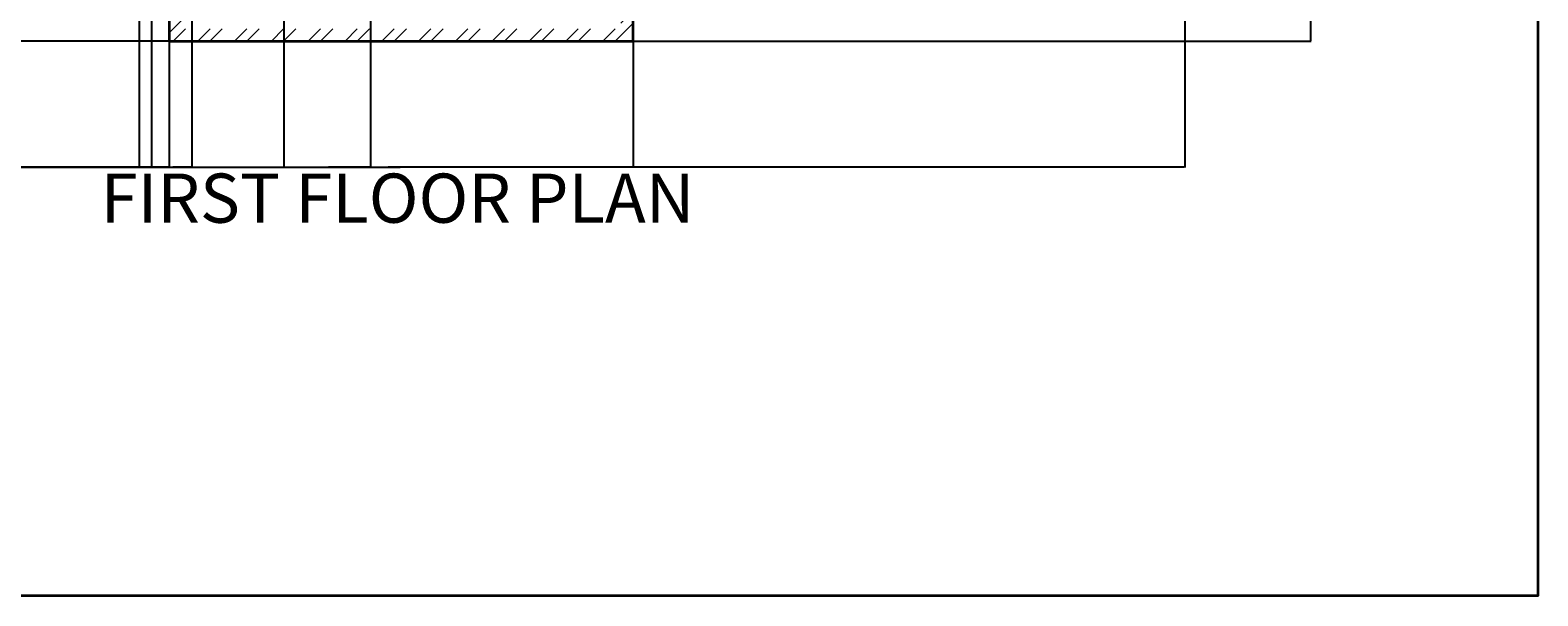
# Model space of a CAD drawing. Units: inches. Extents: x 392 to 1254, y 1207 to 2665.
# Tile 2 of 15: x 702 to 1254, y 1207 to 1414. Entities that reach past the tile are written whole.
import ezdxf

# ---------------------------------------------------------------- set-up
doc = ezdxf.new("R2010")
doc.units = ezdxf.units.IN
for name, color, linetype, lineweight in [('A-ANNO-DIMS', 2, 'Continuous', 18), ('A-ANNO-TEXT', 7, 'Continuous', 25), ('A-ANNO-TTLB', 7, 'Continuous', 35), ('A-WALL', 7, 'Continuous', 35), ('A-WALL-PATT', 252, 'Continuous', 13)]:
    doc.layers.add(name, color=color, linetype=linetype, lineweight=lineweight)
doc.styles.get("Standard").update_dxf_attribs({"font": 'arial.ttf'})
doc.dimstyles.get("Standard").update_dxf_attribs({"dimtxt": 0.18, "dimasz": 0.18, "dimexe": 0.18, "dimexo": 0.0625, "dimgap": 0.09, "dimtad": 0, "dimtih": 1, "dimtoh": 1, "dimdec": 4, "dimzin": 0, "dimdsep": 46, "dimtxsty": 'Standard', "dimcen": 0.09, "dimadec": 0, "dimazin": 0, "dimtfac": 1, "dimtdec": 4, "dimtofl": 0, "dimtmove": 0, "dimatfit": 3, "dimfxl": 1, "dimtolj": 1, "dimtzin": 0, "dimarcsym": 0})

# ---------------------------------------------------------------- blocks, each defined once
blk = doc.blocks.new('*D25')
at = {"layer": 'A-ANNO-DIMS', "color": 0, "lineweight": -2, "transparency": 16777216}
for p, q in [((541.28, 1482.23), (541.28, 1364.02)), ((1124.78, 1482.23), (1124.78, 1364.02)), ((541.46, 1364.2), (832.64, 1364.2)), ((1124.6, 1364.2), (833.43, 1364.2))]:
    blk.add_line(p, q, dxfattribs=at)
at = {"layer": 'A-ANNO-DIMS', "color": 0, "transparency": 16777216}
for points in [[(541.46, 1364.23), (541.46, 1364.17), (541.28, 1364.2)], [(1124.6, 1364.23), (1124.6, 1364.17), (1124.78, 1364.2)]]:
    blk.add_solid(points, dxfattribs=at)
at = {"layer": 'Defpoints', "color": 0, "transparency": 16777216}
for p in [(541.28, 1482.3), (1124.78, 1482.3), (1124.78, 1364.2)]:
    blk.add_point(p, dxfattribs=at)
at = {"layer": 'A-ANNO-DIMS', "color": 0, "transparency": 16777216, "insert": (833.03, 1364.2), "char_height": 0.18, "attachment_point": 5}
blk.add_mtext('\\A1;583.5', dxfattribs=at)
blk = doc.blocks.new('*D26')
at = {"layer": 'A-ANNO-DIMS', "color": 0, "lineweight": -2, "transparency": 16777216}
for p, q in [((541.22, 2229.3), (495, 2229.3)), ((495.18, 2229.12), (495.18, 1819.98)), ((495.18, 1410.48), (495.18, 1819.61)), ((753.23, 1410.3), (495, 1410.3))]:
    blk.add_line(p, q, dxfattribs=at)
at = {"layer": 'A-ANNO-DIMS', "color": 0, "transparency": 16777216}
for points in [[(495.15, 2229.12), (495.21, 2229.12), (495.18, 2229.3)], [(495.15, 1410.48), (495.21, 1410.48), (495.18, 1410.3)]]:
    blk.add_solid(points, dxfattribs=at)
at = {"layer": 'Defpoints', "color": 0, "transparency": 16777216}
for p in [(495.18, 2229.3), (541.28, 2229.3), (753.29, 1410.3)]:
    blk.add_point(p, dxfattribs=at)
at = {"layer": 'A-ANNO-DIMS', "color": 0, "transparency": 16777216, "insert": (495.18, 1819.8), "char_height": 0.18, "attachment_point": 5}
blk.add_mtext('\\A1;819', dxfattribs=at)
blk = doc.blocks.new('*D28')
at = {"layer": 'A-ANNO-DIMS', "color": 0, "lineweight": -2, "transparency": 16777216}
for p, q in [((753.29, 1410.23), (753.29, 1364.02)), ((922.99, 1410.23), (922.99, 1364.02)), ((753.47, 1364.2), (837.75, 1364.2)), ((922.81, 1364.2), (838.52, 1364.2))]:
    blk.add_line(p, q, dxfattribs=at)
at = {"layer": 'A-ANNO-DIMS', "color": 0, "transparency": 16777216}
for points in [[(753.47, 1364.23), (753.47, 1364.17), (753.29, 1364.2)], [(922.81, 1364.23), (922.81, 1364.17), (922.99, 1364.2)]]:
    blk.add_solid(points, dxfattribs=at)
at = {"layer": 'Defpoints', "color": 0, "transparency": 16777216}
for p in [(753.29, 1410.3), (922.99, 1410.3), (922.99, 1364.2)]:
    blk.add_point(p, dxfattribs=at)
at = {"layer": 'A-ANNO-DIMS', "color": 0, "transparency": 16777216, "insert": (838.14, 1364.2), "char_height": 0.18, "attachment_point": 5}
blk.add_mtext('\\A1;169.7', dxfattribs=at)
blk = doc.blocks.new('*D29')
at = {"layer": 'A-ANNO-DIMS', "color": 0, "lineweight": -2, "transparency": 16777216}
for p, q in [((541.28, 1482.23), (541.28, 1364.02)), ((753.29, 1410.23), (753.29, 1364.02)), ((541.46, 1364.2), (647, 1364.2)), ((753.11, 1364.2), (647.57, 1364.2))]:
    blk.add_line(p, q, dxfattribs=at)
at = {"layer": 'A-ANNO-DIMS', "color": 0, "transparency": 16777216}
for points in [[(541.46, 1364.23), (541.46, 1364.17), (541.28, 1364.2)], [(753.11, 1364.23), (753.11, 1364.17), (753.29, 1364.2)]]:
    blk.add_solid(points, dxfattribs=at)
at = {"layer": 'Defpoints', "color": 0, "transparency": 16777216}
for p in [(541.28, 1482.3), (753.29, 1410.3), (753.29, 1364.2)]:
    blk.add_point(p, dxfattribs=at)
at = {"layer": 'A-ANNO-DIMS', "color": 0, "transparency": 16777216, "insert": (647.28, 1364.2), "char_height": 0.18, "attachment_point": 5}
blk.add_mtext('\\A1;212', dxfattribs=at)
blk = doc.blocks.new('*D51')
at = {"layer": 'A-ANNO-DIMS', "color": 0, "lineweight": -2, "transparency": 16777216}
for p, q in [((887.84, 1434.3), (1171.06, 1434.3)), ((1170.88, 1434.12), (1170.88, 1422.48)), ((1170.88, 1410.48), (1170.88, 1422.11)), ((923.05, 1410.3), (1171.06, 1410.3))]:
    blk.add_line(p, q, dxfattribs=at)
at = {"layer": 'A-ANNO-DIMS', "color": 0, "transparency": 16777216}
for points in [[(1170.85, 1434.12), (1170.91, 1434.12), (1170.88, 1434.3)], [(1170.85, 1410.48), (1170.91, 1410.48), (1170.88, 1410.3)]]:
    blk.add_solid(points, dxfattribs=at)
at = {"layer": 'Defpoints', "color": 0, "transparency": 16777216}
for p in [(887.78, 1434.3), (922.99, 1410.3), (1170.88, 1410.3)]:
    blk.add_point(p, dxfattribs=at)
at = {"layer": 'A-ANNO-DIMS', "color": 0, "transparency": 16777216, "insert": (1170.88, 1422.3), "char_height": 0.18, "attachment_point": 5}
blk.add_mtext('\\A1;24', dxfattribs=at)
blk = doc.blocks.new('*D75')
at = {"layer": 'A-ANNO-DIMS', "color": 0, "lineweight": -2, "transparency": 16777216}
for p, q in [((742.28, 2052.23), (742.28, 1364.02)), ((746.78, 2056.73), (746.78, 1364.02)), ((742.46, 1364.2), (744.27, 1364.2)), ((746.6, 1364.2), (744.79, 1364.2))]:
    blk.add_line(p, q, dxfattribs=at)
at = {"layer": 'A-ANNO-DIMS', "color": 0, "transparency": 16777216}
for points in [[(742.46, 1364.23), (742.46, 1364.17), (742.28, 1364.2)], [(746.6, 1364.23), (746.6, 1364.17), (746.78, 1364.2)]]:
    blk.add_solid(points, dxfattribs=at)
at = {"layer": 'Defpoints', "color": 0, "transparency": 16777216}
for p in [(742.28, 2052.3), (746.78, 2056.8), (746.78, 1364.2)]:
    blk.add_point(p, dxfattribs=at)
at = {"layer": 'A-ANNO-DIMS', "color": 0, "transparency": 16777216, "insert": (744.53, 1364.2), "char_height": 0.18, "attachment_point": 5}
blk.add_mtext('\\A1;4.5', dxfattribs=at)
blk = doc.blocks.new('*D78')
at = {"layer": 'A-ANNO-DIMS', "color": 0, "lineweight": -2, "transparency": 16777216}
for p, q in [((746.78, 2056.73), (746.78, 1364.02)), ((761.56, 2056.73), (761.56, 1364.02)), ((746.96, 1364.2), (753.72, 1364.2)), ((761.38, 1364.2), (754.63, 1364.2))]:
    blk.add_line(p, q, dxfattribs=at)
at = {"layer": 'A-ANNO-DIMS', "color": 0, "transparency": 16777216}
for points in [[(746.96, 1364.23), (746.96, 1364.17), (746.78, 1364.2)], [(761.38, 1364.23), (761.38, 1364.17), (761.56, 1364.2)]]:
    blk.add_solid(points, dxfattribs=at)
at = {"layer": 'Defpoints', "color": 0, "transparency": 16777216}
for p in [(746.78, 2056.8), (761.56, 2056.8), (761.56, 1364.2)]:
    blk.add_point(p, dxfattribs=at)
at = {"layer": 'A-ANNO-DIMS', "color": 0, "transparency": 16777216, "insert": (754.17, 1364.2), "char_height": 0.18, "attachment_point": 5}
blk.add_mtext('\\A1;14.782', dxfattribs=at)
blk = doc.blocks.new('*D80')
at = {"layer": 'A-ANNO-DIMS', "color": 0, "lineweight": -2, "transparency": 16777216}
for p, q in [((795.21, 2052.23), (795.21, 1364.02)), ((826.91, 2052.23), (826.91, 1364.02)), ((795.39, 1364.2), (810.6, 1364.2)), ((826.73, 1364.2), (811.52, 1364.2))]:
    blk.add_line(p, q, dxfattribs=at)
at = {"layer": 'A-ANNO-DIMS', "color": 0, "transparency": 16777216}
for points in [[(795.39, 1364.23), (795.39, 1364.17), (795.21, 1364.2)], [(826.73, 1364.23), (826.73, 1364.17), (826.91, 1364.2)]]:
    blk.add_solid(points, dxfattribs=at)
at = {"layer": 'Defpoints', "color": 0, "transparency": 16777216}
for p in [(795.21, 2052.3), (826.91, 2052.3), (826.91, 1364.2)]:
    blk.add_point(p, dxfattribs=at)
at = {"layer": 'A-ANNO-DIMS', "color": 0, "transparency": 16777216, "insert": (811.06, 1364.2), "char_height": 0.18, "attachment_point": 5}
blk.add_mtext('\\A1;31.694', dxfattribs=at)

msp = doc.modelspace()

# ---------------------------------------------------------------- hatches: boundary and pattern name
at = {"layer": 'A-WALL-PATT'}
h = msp.add_hatch(dxfattribs=at)
h.set_pattern_fill('ANSI32', color=256)
h.paths.add_polyline_path([(579.5309, 2227.0453), (579.5309, 2229.2953), (541.2807, 2229.2953), (541.2807, 2182.3091), (545.7807, 2182.3091), (545.7807, 2224.7953), (579.5309, 2224.7953)])
h.paths.add_polyline_path([(655.4442, 2229.2953), (627.5309, 2229.2953), (627.5309, 2224.7953), (655.4442, 2224.7953), (655.4442, 2227.0453)])
h.paths.add_polyline_path([(703.0758, 2229.2953), (678.5257, 2229.2953), (678.5257, 2227.0453), (678.5257, 2224.7953), (689.7807, 2224.7953), (689.7807, 2158.6973), (694.2807, 2158.6973), (694.2807, 2224.7953), (703.0758, 2224.7953)])
h.paths.add_polyline_path([(768.5767, 2229.2953), (727.0758, 2229.2953), (727.0758, 2224.7953), (742.2807, 2224.7953), (742.2807, 2128.7953), (694.2807, 2128.7953), (694.2807, 2134.0554), (689.7807, 2134.0554), (689.7807, 2090.2854), (694.2807, 2090.2854), (694.2807, 2124.2953), (742.2807, 2124.2953), (742.2807, 2052.2953), (795.2123, 2052.2953), (795.2123, 2054.5453), (795.2123, 2056.7953), (746.7807, 2056.7953), (746.7807, 2224.7953), (768.5767, 2224.7953)])
h.paths.add_polyline_path([(867.5089, 2229.2953), (804.5767, 2229.2953), (804.5767, 2224.7953), (830.7807, 2224.7953), (830.7807, 2056.7953), (826.9066, 2056.7953), (826.9066, 2052.2953), (830.7807, 2052.2953), (830.7807, 1886.6777, -0.01766664), (830.8602, 1884.2953), (835.0818, 1884.2953, -0.04411348), (835.2807, 1889.9369), (835.2807, 2052.2953), (839.418, 2052.2953), (839.418, 2056.7953), (835.2807, 2056.7953), (835.2807, 2224.7953), (867.5089, 2224.7953)])
h.paths.add_polyline_path([(939.8604, 2229.2953), (903.5089, 2229.2953), (903.5089, 2227.0453), (903.5089, 2224.7953), (919.2807, 2224.7953), (919.2807, 2056.7953), (870.6499, 2056.7953), (870.6499, 2052.2953), (923.7807, 2052.2953), (923.7807, 2124.2953), (971.7807, 2124.2953), (971.7807, 2089.7112), (974.0307, 2089.7112), (976.2807, 2089.7112), (976.2807, 2133.56), (974.0307, 2133.56), (971.7807, 2133.56), (971.7807, 2128.7953), (923.7807, 2128.7953), (923.7807, 2224.7953), (939.8604, 2224.7953)])
h.paths.add_polyline_path([(1124.7807, 2229.2953), (1009.403, 2229.2953), (1009.403, 2224.7953), (1120.2807, 2224.7953), (1120.2807, 2184.7605), (1124.7807, 2184.7605)])
h.paths.add_polyline_path([(1124.7807, 2124.7605), (1120.2807, 2124.7605), (1120.2807, 2056.7953), (976.2807, 2056.7953), (976.2807, 2061.471), (971.7807, 2061.471), (971.7807, 2047.7483), (974.0307, 2047.7483), (976.2807, 2047.7483), (976.2807, 2052.2953), (1120.2807, 2052.2953), (1120.2807, 1992.457), (1124.7807, 1992.457)])
h.paths.add_polyline_path([(1124.7807, 1932.457), (1122.5307, 1932.457), (1120.2807, 1932.457), (1120.2807, 1884.2953), (976.2807, 1884.2953), (976.2807, 2019.9536), (971.7807, 2019.9536), (971.7807, 1884.2953), (869.0911, 1884.2953), (869.0911, 1879.7953), (971.7807, 1879.7953), (1013.7807, 1879.7953), (1013.7807, 1831.7953), (971.7807, 1831.7953), (971.7807, 1822.3831), (974.0307, 1822.3831), (976.2807, 1822.3831), (976.2807, 1827.2953), (1013.7807, 1827.2953), (1025.6191, 1827.2953), (1025.6191, 1829.5453), (1025.6191, 1831.7953), (1018.2807, 1831.7953), (1018.2807, 1879.7953), (1120.2807, 1879.7953), (1120.2807, 1866.9192), (1124.7807, 1866.9192)])
h.paths.add_polyline_path([(1124.7807, 1842.9192), (1122.5307, 1842.9192), (1120.2807, 1842.9192), (1120.2807, 1831.7953), (1050.2021, 1831.7953), (1050.2021, 1827.2953), (1120.2807, 1827.2953), (1120.2807, 1781.4559), (1124.7807, 1781.4559)])
h.paths.add_polyline_path([(976.2807, 1790.8718), (971.7807, 1790.8718), (971.7807, 1648.3339), (976.2807, 1648.3339), (976.2807, 1654.7953), (1120.2807, 1654.7953), (1120.2807, 1626.3807), (1124.7807, 1626.3807), (1124.7807, 1721.4559), (1120.2807, 1721.4559), (1120.2807, 1659.2953), (976.2807, 1659.2953)])
h.paths.add_polyline_path([(1124.7807, 1566.3807), (1120.2807, 1566.3807), (1120.2807, 1486.7953), (1101.07, 1486.7953), (1101.07, 1482.2953), (1124.7807, 1482.2953)])
h.paths.add_polyline_path([(1041.07, 1484.5453), (1041.07, 1486.7953), (1006.2807, 1486.7953), (1006.2807, 1484.5453), (1006.2807, 1482.2953), (1041.07, 1482.2953)])
h.paths.add_polyline_path([(976.2807, 1617.5497), (974.0307, 1617.5497), (971.7807, 1617.5497), (971.7807, 1599.2953), (965.8041, 1599.2953), (965.8041, 1594.7953), (971.7807, 1594.7953), (971.7807, 1486.7953), (954.1249, 1486.7953), (954.1249, 1482.2953), (981.5717, 1482.2953), (981.5717, 1484.5453), (981.5717, 1486.7953), (976.2807, 1486.7953)])
h.paths.add_polyline_path([(930.1249, 1486.7953), (887.7807, 1486.7953), (887.7807, 1594.7953), (941.9141, 1594.7953), (941.9141, 1597.0453), (941.9141, 1599.2953), (887.7807, 1599.2953), (887.7807, 1659.2953), (863.5916, 1659.2953), (863.5916, 1654.7953), (883.2807, 1654.7953), (883.2807, 1438.7953), (782.7807, 1438.7953), (782.7807, 1486.7953), (782.7807, 1654.7953), (800.1309, 1654.7953), (800.1309, 1657.0453), (800.1309, 1659.2953), (778.2807, 1659.2953), (778.2807, 1599.2953), (721.7333, 1599.2953), (721.7333, 1597.0453), (721.7333, 1594.7953), (778.2807, 1594.7953), (778.2807, 1486.7953), (729.598, 1486.7953), (729.598, 1482.2953), (753.2885, 1482.2953), (753.2885, 1410.2953), (922.9852, 1410.2953), (922.9852, 1482.2953), (930.1249, 1482.2953)])
h.paths.add_polyline_path([(918.4852, 1482.2953), (918.4852, 1414.7953), (757.7885, 1414.7953), (757.7885, 1482.2953), (778.2807, 1482.2953), (778.2807, 1434.2953), (782.7807, 1434.2953), (887.7807, 1434.2953), (887.7807, 1438.7953), (887.7807, 1482.2953)], flags=16)
h.paths.add_polyline_path([(694.2807, 1594.7953), (700.4169, 1594.7953), (700.4169, 1597.0453), (700.4169, 1599.2953), (694.2807, 1599.2953), (694.2807, 1617.7503), (692.0307, 1617.7503), (689.7807, 1617.7503), (689.7807, 1486.7953), (682.7672, 1486.7953), (682.7672, 1482.2953), (705.598, 1482.2953), (705.598, 1484.5453), (705.598, 1486.7953), (694.2807, 1486.7953)])
h.paths.add_polyline_path([(545.7807, 1654.7953), (689.7807, 1654.7953), (689.7807, 1649.7691), (694.2807, 1649.7691), (694.2807, 1789.3981), (692.0307, 1789.3981), (689.7807, 1789.3981), (689.7807, 1659.2953), (545.7807, 1659.2953), (545.7807, 1714.4681), (543.5307, 1714.4681), (541.2807, 1714.4681), (541.2807, 1482.2953), (567.0628, 1482.2953), (567.0628, 1484.5453), (567.0628, 1486.7953), (545.7807, 1486.7953)])
h.paths.add_polyline_path([(545.7807, 1827.2953), (620.2247, 1827.2953), (620.2247, 1829.5453), (620.2247, 1831.7953), (545.7807, 1831.7953), (545.7807, 1846.8518), (541.2807, 1846.8518), (541.2807, 1774.4681), (545.7807, 1774.4681)])
h.paths.add_polyline_path([(797.0944, 1884.2953), (694.2807, 1884.2953), (694.2807, 2019.0288), (692.0307, 2019.0288), (689.7807, 2019.0288), (689.7807, 1884.2953), (545.7807, 1884.2953), (545.7807, 1951.8244), (541.2807, 1951.8244), (541.2807, 1870.8518), (543.5307, 1870.8518), (545.7807, 1870.8518), (545.7807, 1879.7953), (647.7807, 1879.7953), (647.7807, 1831.7953), (642.6413, 1831.7953), (642.6413, 1827.2953), (652.2807, 1827.2953), (689.7807, 1827.2953), (689.7807, 1821.0531), (694.2807, 1821.0531), (694.2807, 1831.7953), (652.2807, 1831.7953), (652.2807, 1879.7953), (797.0944, 1879.7953), (797.0944, 1882.0453)])
h.paths.add_polyline_path([(545.7807, 2122.3091), (541.2807, 2122.3091), (541.2807, 2011.8244), (543.5307, 2011.8244), (545.7807, 2011.8244), (545.7807, 2052.2953), (689.7807, 2052.2953), (689.7807, 2048.2048), (694.2807, 2048.2048), (694.2807, 2061.3129), (692.0307, 2061.3129), (689.7807, 2061.3129), (689.7807, 2056.7953), (545.7807, 2056.7953)])

# ---------------------------------------------------------------- linework, layer by layer
at = {"layer": 'A-ANNO-TTLB'}
msp.add_lwpolyline([(391.939, 2664.8979), (1253.97, 2664.8979), (1253.97, 1207.2611), (391.939, 1207.2611)], close=True, dxfattribs=at)
at = {"layer": 'A-WALL'}
for p, q in [((753.2885, 1482.2953), (753.2885, 1410.2953)), ((922.9852, 1410.2953), (922.9852, 1482.2953)), ((753.2885, 1410.2953), (922.9852, 1410.2953))]:
    msp.add_line(p, q, dxfattribs=at)

# ---------------------------------------------------------------- texts
at = {"layer": 'A-ANNO-TEXT', "insert": (728.2019, 1361.8565), "char_height": 18, "attachment_point": 1}
msp.add_mtext_dynamic_manual_height_columns('FIRST FLOOR PLAN ', width=500.372474, gutter_width=12.5, heights=[0], dxfattribs=at)

# ---------------------------------------------------------------- dimensions: what is measured, and where the dimension line sits
at = {"layer": 'A-ANNO-DIMS'}
for base, p1, p2, picture, middle in [((495.1807, 2229.2953), (753.2885, 1410.2953), (541.2807, 2229.2953), '*D26', (495.1807, 1819.7953)), ((1170.8807, 1410.2953), (887.7807, 1434.2953), (922.9852, 1410.2953), '*D51', (1170.8807, 1422.2953))]:
    dim = msp.add_linear_dim(base=base, p1=p1, p2=p2, angle=90, dimstyle='Standard', override={"dimdec": 0, "dimlfac": 1, "dimrnd": 0, "dimzin": 0, "dimdsep": 46, "dimlunit": 2}, dxfattribs=at)
    dim.commit()
    dim.dimension.update_dxf_attribs({"geometry": picture, "text_midpoint": middle})
for base, p1, p2, override, picture, middle in [((746.7807, 1364.1953), (742.2807, 2052.2953), (746.7807, 2056.7953), {"dimdec": 1, "dimlfac": 1, "dimrnd": 0, "dimzin": 0, "dimdsep": 46, "dimlunit": 2}, '*D75', (744.5307, 1364.1953)), ((761.5625, 1364.1953), (746.7807, 2056.7953), (761.5625, 2056.7953), {"dimdec": 3, "dimlfac": 1, "dimrnd": 0, "dimzin": 0, "dimdsep": 46, "dimlunit": 2}, '*D78', (754.1716, 1364.1953)), ((826.9066, 1364.1953), (795.2123, 2052.2953), (826.9066, 2052.2953), {"dimdec": 3, "dimlfac": 1, "dimrnd": 0, "dimzin": 0, "dimdsep": 46, "dimlunit": 2}, '*D80', (811.0595, 1364.1953)), ((1124.7807, 1364.1953), (541.2807, 1482.2953), (1124.7807, 1482.2953), {"dimdec": 1, "dimlfac": 1, "dimrnd": 0, "dimzin": 0, "dimdsep": 46, "dimlunit": 2}, '*D25', (833.0307, 1364.1953)), ((753.2885, 1364.1953), (541.2807, 1482.2953), (753.2885, 1410.2953), {"dimdec": 0, "dimlfac": 1, "dimrnd": 0, "dimzin": 0, "dimdsep": 46, "dimlunit": 2}, '*D29', (647.2846, 1364.1953)), ((922.9852, 1364.1953), (753.2885, 1410.2953), (922.9852, 1410.2953), {"dimdec": 1, "dimlfac": 1, "dimrnd": 0, "dimzin": 0, "dimdsep": 46, "dimlunit": 2}, '*D28', (838.1369, 1364.1953))]:
    dim = msp.add_linear_dim(base=base, p1=p1, p2=p2, dimstyle='Standard', override=override, dxfattribs=at)
    dim.commit()
    dim.dimension.update_dxf_attribs({"geometry": picture, "text_midpoint": middle})

doc.saveas('drawing.dxf')
